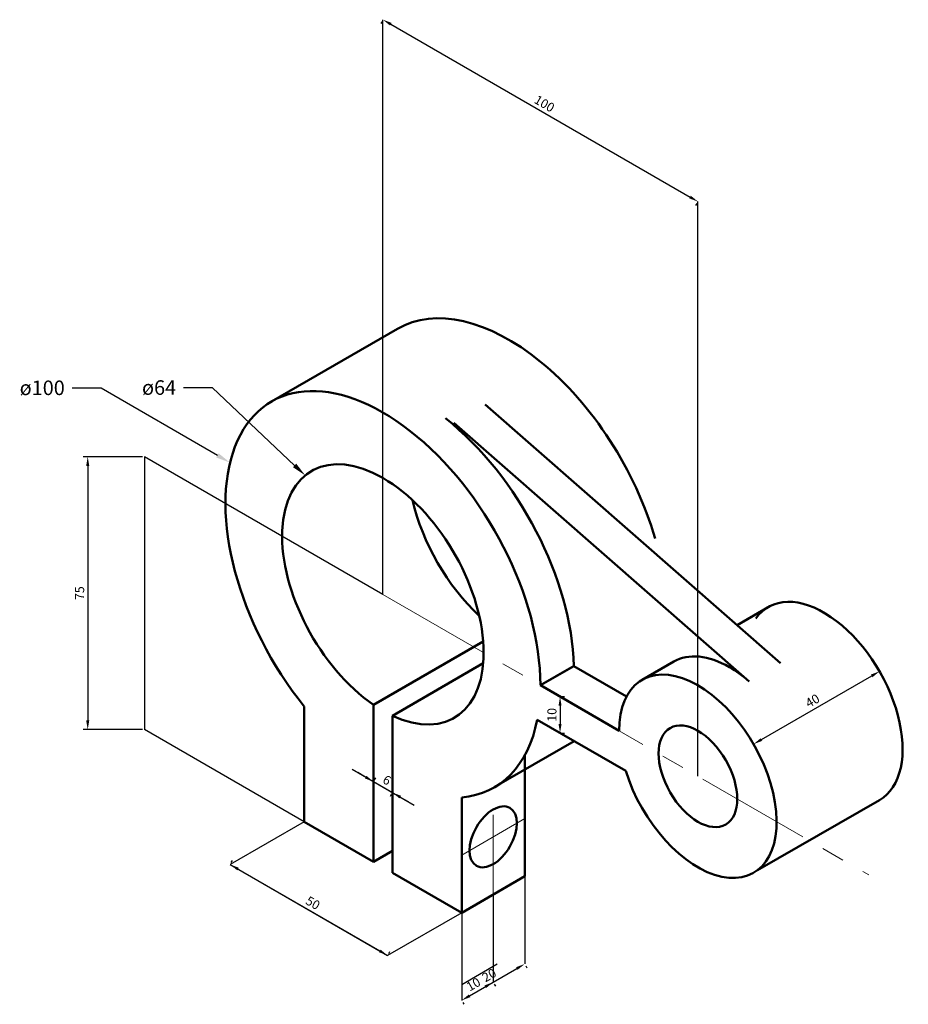
# Model space of a CAD drawing. Units: millimetres. Extents: x 1851 to 2096, y 1528 to 1798.
import ezdxf
from ezdxf import colors
from ezdxf.entities.mleader import LeaderData, LeaderLine
from ezdxf.math import Vec2, Vec3

# ---------------------------------------------------------------- set-up
doc = ezdxf.new("R2010")
doc.units = ezdxf.units.MM
doc.linetypes.add('CENTER', pattern=[50.8, 31.75, -6.35, 6.35, -6.35])
for name, color, linetype, lineweight in [('M-CNTR', 1, 'CENTER', 18), ('M-DIMS', 2, 'Continuous', 25), ('M-OUTL', 7, 'Continuous', 50), ('M-TEXT', 3, 'Continuous', 25)]:
    doc.layers.add(name, color=color, linetype=linetype, lineweight=lineweight)
doc.styles.get("Standard").update_dxf_attribs({"font": 'arial.ttf'})
doc.dimstyles.new('ISO-25', dxfattribs={"dimtxt": 2.5, "dimasz": 2.5, "dimexe": 1.25, "dimexo": 0.625, "dimtad": 1, "dimtxsty": 'Standard', "dimcen": 2.5, "dimadec": 0, "dimazin": 0, "dimtfac": 1, "dimtmove": 0, "dimatfit": 3, "dimfxl": 1, "dimarcsym": 0})

# ---------------------------------------------------------------- blocks, each defined once
blk = doc.blocks.new('*D1')
at = {"layer": 'Defpoints', "color": 0, "transparency": 16777216}
for p in [(2087.65, 1619.14), (2087.65, 1619.14), (2053.01, 1599.14)]:
    blk.add_point(p, dxfattribs=at)
at = {"layer": 'M-DIMS', "color": 0, "lineweight": -2, "transparency": 16777216}
for p, q in [((2087.97, 1618.59), (2088.28, 1618.05)), ((2055.18, 1600.39), (2085.49, 1617.89)), ((2053.33, 1598.59), (2053.64, 1598.05))]:
    blk.add_line(p, q, dxfattribs=at)
at = {"layer": 'M-DIMS', "color": 0, "transparency": 16777216}
for points in [[(2085.28, 1618.25), (2085.7, 1617.52), (2087.65, 1619.14)], [(2054.97, 1600.75), (2055.39, 1600.02), (2053.01, 1599.14)]]:
    blk.add_solid(points, dxfattribs=at)
at = {"layer": 'M-DIMS', "color": 0, "transparency": 16777216, "insert": (2069.38, 1610.78), "char_height": 2.5, "attachment_point": 5, "rotation": 30}
blk.add_mtext('40', dxfattribs=at)
blk = doc.blocks.new('*D2')
at = {"layer": 'Defpoints', "color": 0, "transparency": 16777216}
for p in [(1948.5, 1588.82), (1953.7, 1585.82), (1953.7, 1585.82)]:
    blk.add_point(p, dxfattribs=at)
at = {"layer": 'M-DIMS', "color": 0, "lineweight": -2, "transparency": 16777216}
for p, q in [((1946.34, 1590.07), (1944.17, 1591.32)), ((1948.5, 1588.82), (1953.7, 1585.82)), ((1948.82, 1589.36), (1949.13, 1589.91)), ((1953.39, 1585.28), (1953.07, 1584.74)), ((1955.86, 1584.57), (1958.03, 1583.32))]:
    blk.add_line(p, q, dxfattribs=at)
at = {"layer": 'M-DIMS', "color": 0, "transparency": 16777216}
for points in [[(1946.55, 1590.43), (1946.13, 1589.71), (1948.5, 1588.82)], [(1956.07, 1584.93), (1955.66, 1584.21), (1953.7, 1585.82)]]:
    blk.add_solid(points, dxfattribs=at)
at = {"layer": 'M-DIMS', "color": 0, "transparency": 16777216, "insert": (1952.05, 1588.97), "char_height": 2.5, "attachment_point": 5, "rotation": 330}
blk.add_mtext('6', dxfattribs=at)
blk = doc.blocks.new('*D3')
at = {"layer": 'Defpoints', "color": 0, "transparency": 16777216}
for p in [(1999.8, 1612.18), (1999.8, 1602.18), (1999.8, 1602.18)]:
    blk.add_point(p, dxfattribs=at)
at = {"layer": 'M-DIMS', "color": 0, "lineweight": -2, "transparency": 16777216}
for p, q in [((2000.42, 1612.18), (2001.05, 1612.18)), ((1999.8, 1609.68), (1999.8, 1604.68)), ((2000.42, 1602.18), (2001.05, 1602.18))]:
    blk.add_line(p, q, dxfattribs=at)
at = {"layer": 'M-DIMS', "color": 0, "transparency": 16777216}
for points in [[(1999.38, 1609.68), (2000.21, 1609.68), (1999.8, 1612.18)], [(1999.38, 1604.68), (2000.21, 1604.68), (1999.8, 1602.18)]]:
    blk.add_solid(points, dxfattribs=at)
at = {"layer": 'M-DIMS', "color": 0, "transparency": 16777216, "insert": (1997.89, 1607.18), "char_height": 2.5, "attachment_point": 5, "rotation": 90}
blk.add_mtext('10', dxfattribs=at)
blk = doc.blocks.new('*D4')
at = {"layer": 'Defpoints', "color": 0, "transparency": 16777216}
for p in [(1885.58, 1678.13), (1869.92, 1603.13), (1885.58, 1603.13)]:
    blk.add_point(p, dxfattribs=at)
at = {"layer": 'M-DIMS', "color": 0, "lineweight": -2, "transparency": 16777216}
for p, q in [((1884.95, 1678.13), (1868.67, 1678.13)), ((1869.92, 1675.63), (1869.92, 1605.63)), ((1884.95, 1603.13), (1868.67, 1603.13))]:
    blk.add_line(p, q, dxfattribs=at)
at = {"layer": 'M-DIMS', "color": 0, "transparency": 16777216}
for points in [[(1869.5, 1675.63), (1870.34, 1675.63), (1869.92, 1678.13)], [(1869.5, 1605.63), (1870.34, 1605.63), (1869.92, 1603.13)]]:
    blk.add_solid(points, dxfattribs=at)
at = {"layer": 'M-DIMS', "color": 0, "transparency": 16777216, "insert": (1868.02, 1640.63), "char_height": 2.5, "attachment_point": 5, "rotation": 90}
blk.add_mtext('75', dxfattribs=at)
blk = doc.blocks.new('*D5')
at = {"layer": 'Defpoints', "color": 0, "transparency": 16777216}
for p in [(1909.09, 1566.04), (1952.39, 1541.04), (1952.39, 1541.04)]:
    blk.add_point(p, dxfattribs=at)
at = {"layer": 'M-DIMS', "color": 0, "lineweight": -2, "transparency": 16777216}
for p, q in [((1909.4, 1566.58), (1909.71, 1567.12)), ((1911.25, 1564.79), (1950.22, 1542.29)), ((1952.7, 1541.58), (1953.01, 1542.12))]:
    blk.add_line(p, q, dxfattribs=at)
at = {"layer": 'M-DIMS', "color": 0, "transparency": 16777216}
for points in [[(1911.46, 1565.15), (1911.04, 1564.43), (1909.09, 1566.04)], [(1950.43, 1542.65), (1950.01, 1541.93), (1952.39, 1541.04)]]:
    blk.add_solid(points, dxfattribs=at)
at = {"layer": 'M-DIMS', "color": 0, "transparency": 16777216, "insert": (1931.69, 1555.19), "char_height": 2.5, "attachment_point": 5, "rotation": 330}
blk.add_mtext('50', dxfattribs=at)
blk = doc.blocks.new('*D6')
at = {"layer": 'Defpoints', "color": 0, "transparency": 16777216}
for p in [(1990.07, 1538.69), (1990.07, 1538.69), (1972.75, 1528.69)]:
    blk.add_point(p, dxfattribs=at)
at = {"layer": 'M-DIMS', "color": 0, "lineweight": -2, "transparency": 16777216}
for p, q in [((1974.92, 1529.94), (1987.91, 1537.44)), ((1990.38, 1538.15), (1990.7, 1537.61)), ((1973.06, 1528.15), (1973.38, 1527.61))]:
    blk.add_line(p, q, dxfattribs=at)
at = {"layer": 'M-DIMS', "color": 0, "transparency": 16777216}
for points in [[(1987.7, 1537.8), (1988.12, 1537.08), (1990.07, 1538.69)], [(1974.71, 1530.3), (1975.13, 1529.58), (1972.75, 1528.69)]]:
    blk.add_solid(points, dxfattribs=at)
at = {"layer": 'M-DIMS', "color": 0, "transparency": 16777216, "insert": (1980.46, 1535.34), "char_height": 2.5, "attachment_point": 5, "rotation": 30}
blk.add_mtext('20', dxfattribs=at)
blk = doc.blocks.new('*D7')
at = {"layer": 'Defpoints', "color": 0, "transparency": 16777216}
for p in [(1981.41, 1533.69), (1981.41, 1533.69), (1972.75, 1528.69)]:
    blk.add_point(p, dxfattribs=at)
at = {"layer": 'M-DIMS', "color": 0, "lineweight": -2, "transparency": 16777216}
for p, q in [((1974.92, 1529.94), (1979.25, 1532.44)), ((1981.72, 1533.15), (1982.04, 1532.61)), ((1973.06, 1528.15), (1973.38, 1527.61))]:
    blk.add_line(p, q, dxfattribs=at)
at = {"layer": 'M-DIMS', "color": 0, "transparency": 16777216}
for points in [[(1979.04, 1532.8), (1979.46, 1532.08), (1981.41, 1533.69)], [(1974.71, 1530.3), (1975.13, 1529.58), (1972.75, 1528.69)]]:
    blk.add_solid(points, dxfattribs=at)
at = {"layer": 'M-DIMS', "color": 0, "transparency": 16777216, "insert": (1976.13, 1532.84), "char_height": 2.5, "attachment_point": 5, "rotation": 30}
blk.add_mtext('10', dxfattribs=at)
blk = doc.blocks.new('*D8')
at = {"layer": 'Defpoints', "color": 0, "transparency": 16777216}
for p in [(1951.1, 1798.28), (2037.7, 1748.28), (2037.7, 1748.28)]:
    blk.add_point(p, dxfattribs=at)
at = {"layer": 'M-DIMS', "color": 0, "lineweight": -2, "transparency": 16777216}
for p, q in [((1950.79, 1797.73), (1950.48, 1797.19)), ((1953.27, 1797.03), (2035.54, 1749.53)), ((2037.39, 1747.73), (2037.08, 1747.19))]:
    blk.add_line(p, q, dxfattribs=at)
at = {"layer": 'M-DIMS', "color": 0, "transparency": 16777216}
for points in [[(1953.47, 1797.39), (1953.06, 1796.66), (1951.1, 1798.28)], [(2035.75, 1749.89), (2035.33, 1749.16), (2037.7, 1748.28)]]:
    blk.add_solid(points, dxfattribs=at)
at = {"layer": 'M-DIMS', "color": 0, "transparency": 16777216, "insert": (1995.35, 1774.92), "char_height": 2.5, "attachment_point": 5, "rotation": 330}
blk.add_mtext('100', dxfattribs=at)

msp = doc.modelspace()

# ---------------------------------------------------------------- linework, layer by layer
at = {"layer": 'M-CNTR'}
for p, q in [((1951.101, 1640.297), (2084.688, 1563.17)), ((1972.752, 1568.646), (1990.072, 1578.646)), ((1981.412, 1557.797), (1981.412, 1579.687))]:
    msp.add_line(p, q, dxfattribs=at)
at = {"layer": 'M-DIMS'}
for p, q in [((1951.101, 1749.048), (1951.101, 1798.276)), ((1951.101, 1640.297), (1951.101, 1749.048)), ((2037.704, 1699.048), (2037.704, 1748.276)), ((2037.704, 1590.297), (2037.704, 1699.048)), ((1951.101, 1640.297), (1885.578, 1678.127)), ((1885.578, 1678.127), (1885.578, 1603.127)), ((1929.45, 1577.797), (1885.578, 1603.127)), ((1942.611, 1592.225), (1959.69, 1582.364)), ((1929.45, 1577.797), (1909.085, 1566.039)), ((1909.085, 1566.039), (1952.387, 1541.039)), ((1990.072, 1562.797), (1990.072, 1538.692)), ((1981.412, 1557.797), (1981.412, 1533.692)), ((1972.752, 1552.797), (1952.387, 1541.039)), ((1972.752, 1552.797), (1972.752, 1528.692)), ((1972.752, 1533.084), (1982.547, 1538.739))]:
    msp.add_line(p, q, dxfattribs=at)
at = {"layer": 'M-OUTL'}
for p, q in [((1920.482, 1693.33), (1955.123, 1713.33)), ((2060.437, 1621.378), (1979.247, 1692.459)), ((2051.777, 1616.378), (1970.587, 1687.459)), ((2048.461, 1631.863), (2057.035, 1636.814)), ((1948.503, 1609.938), (1978.692, 1627.367)), ((1953.699, 1606.938), (1978.692, 1621.367)), ((2022.394, 1616.814), (2031.055, 1621.814)), ((1994.402, 1615.297), (2003.597, 1620.605)), ((1994.402, 1615.297), (2003.063, 1620.297)), ((2003.597, 1620.605), (2018.102, 1612.23)), ((1994.402, 1615.297), (2016.053, 1602.797)), ((1929.45, 1577.797), (1929.45, 1609.495)), ((1948.503, 1591.887), (1948.503, 1609.938)), ((1953.699, 1588.887), (1953.699, 1606.938)), ((1993.527, 1605.802), (2017.86, 1591.753)), ((1981.72, 1587.264), (2003.678, 1599.942)), ((1990.072, 1562.797), (1990.072, 1596.002)), ((1948.503, 1591.887), (1948.503, 1566.797)), ((1953.699, 1588.887), (1953.699, 1563.797)), ((1972.752, 1552.797), (1972.752, 1584.495)), ((2054.053, 1564.468), (2087.637, 1583.77)), ((1948.503, 1566.797), (1929.45, 1577.797)), ((1929.45, 1577.797), (1948.503, 1566.797)), ((1948.503, 1566.797), (1953.699, 1569.797)), ((1953.699, 1563.797), (1972.752, 1552.797)), ((1972.752, 1552.797), (1990.072, 1562.797))]:
    msp.add_line(p, q, dxfattribs=at)
for centre, major_axis, start_param, end_param in [((1985.742, 1660.297), (30.619, -53.033), 7.4496374, 9.424778), ((1951.101, 1640.297), (30.619, -53.033), 7.0685835, 11.2573737), ((1960.312, 1644.189), (30.619, -53.033), 7.0967055, 8.4532717), ((1951.101, 1640.297), (19.596, -33.941), 5.591675, 11.6870846), ((1985.742, 1660.297), (19.596, -33.941), 4.225694, 5.1990839), ((2072.345, 1610.297), (15.309, -26.517), 6.2820534, 9.6831645), ((2046.364, 1595.297), (15.309, -26.517), 2.3561945, 3.1415927), ((2037.704, 1590.297), (15.309, -26.517), 4.3385077, 10.2101761), ((2046.364, 1595.297), (15.309, -26.517), 2.1035142, 2.3561945), ((1951.101, 1640.297), (30.619, -53.033), 6.0213859, 6.8672255)]:
    msp.add_ellipse(centre, major_axis=major_axis, ratio=0.5773503, start_param=start_param, end_param=end_param, dxfattribs=at)
for centre, major_axis in [((2037.704, 1590.297), (7.655, -13.258)), ((1981.412, 1573.646), (-4.593, -7.955))]:
    msp.add_ellipse(centre, major_axis=major_axis, ratio=0.5773503, dxfattribs=at)

# ---------------------------------------------------------------- dimensions: what is measured, and where the dimension line sits
at = {"layer": 'M-DIMS'}
for base, p1, p2, angle, picture, middle in [((2037.704, 1748.276), (1951.101, 1798.276), (2037.704, 1748.276), 330, '*D8', (1995.353, 1774.922)), ((1869.92, 1603.127), (1885.578, 1678.127), (1885.578, 1603.127), 270, '*D4', (1868.023, 1640.627)), ((1952.387, 1541.039), (1909.085, 1566.039), (1952.387, 1541.039), 330, '*D5', (1931.687, 1555.186)), ((1990.072, 1538.692), (1972.752, 1528.692), (1990.072, 1538.692), 30, '*D6', (1980.461, 1535.339)), ((1981.412, 1533.692), (1972.752, 1528.692), (1981.412, 1533.692), 30, '*D7', (1976.131, 1532.839))]:
    dim = msp.add_linear_dim(base=base, p1=p1, p2=p2, angle=angle, dimstyle='ISO-25', override={"dimrnd": 0}, dxfattribs=at)
    dim.commit()
    dim.dimension.update_dxf_attribs({"geometry": picture, "text_midpoint": middle})
for p1, p2, picture, middle in [((2053.013, 1599.136), (2087.654, 1619.136), '*D1', (2069.383, 1610.782)), ((1999.796, 1612.182), (1999.796, 1602.182), '*D3', (1997.895, 1607.182)), ((1948.503, 1588.823), (1953.699, 1585.823), '*D2', (1952.052, 1588.97))]:
    dim = msp.add_aligned_dim(p1=p1, p2=p2, distance=0, dimstyle='ISO-25', override={"dimclrd": 0, "dimclre": 0, "dimclrt": 0}, dxfattribs=at)
    dim.commit()
    dim.dimension.update_dxf_attribs({"geometry": picture, "text_midpoint": middle})

# ---------------------------------------------------------------- leaders
at = {"layer": 'M-TEXT'}
ml = msp.add_multileader_mtext('Standard', dxfattribs=at)
ml.set_content('ø100', color=256)
ml.set_leader_properties()
ml.build(insert=Vec2(0, 0))
ctx = ml.context
ctx.base_point, ctx.plane_origin = Vec3(1849.491, 1696.974), Vec3(1909.052, 1676.511)
ctx.text_align_type = 2
notes = []
notes.append((ctx, [(0, (1, 1, 0), (1873.609, 1696.974), (-1, 0), 8, [(0, [(1909.052, 1676.511)], 0, [])])]))
ctx.mtext.insert, ctx.mtext.alignment, ctx.mtext.flow_direction = Vec3(1863.609, 1699.082), 3, 5
ml = msp.add_multileader_mtext('Standard', dxfattribs=at)
ml.set_content('ø64', color=256)
ml.set_leader_properties()
ml.build(insert=Vec2(0, 0))
ctx = ml.context
ctx.base_point, ctx.plane_origin = Vec3(1883.217, 1697.048), Vec3(1929.726, 1673.005)
ctx.text_align_type = 2
notes.append((ctx, [(0, (1, 1, 0), (1904.224, 1697.048), (-1, 0), 8, [(0, [(1929.726, 1673.005)], 0, [])])]))
ctx.mtext.insert, ctx.mtext.alignment, ctx.mtext.flow_direction = Vec3(1894.224, 1699.156), 3, 5
for ctx, leaders in notes:
    for number, flags, end, landing, length, lines in leaders:
        leader = LeaderData()
        leader.index, (leader.has_last_leader_line, leader.has_dogleg_vector, leader.attachment_direction) = number, flags
        leader.last_leader_point, leader.dogleg_vector, leader.dogleg_length = Vec3(end), Vec3(landing), length
        for number, points, colour, breaks in lines:
            line = LeaderLine()
            line.index, line.vertices, line.color, line.breaks = number, Vec3.list(points), colors.encode_raw_color(colour), breaks
            leader.lines.append(line)
        ctx.leaders.append(leader)

doc.saveas('drawing.dxf')
